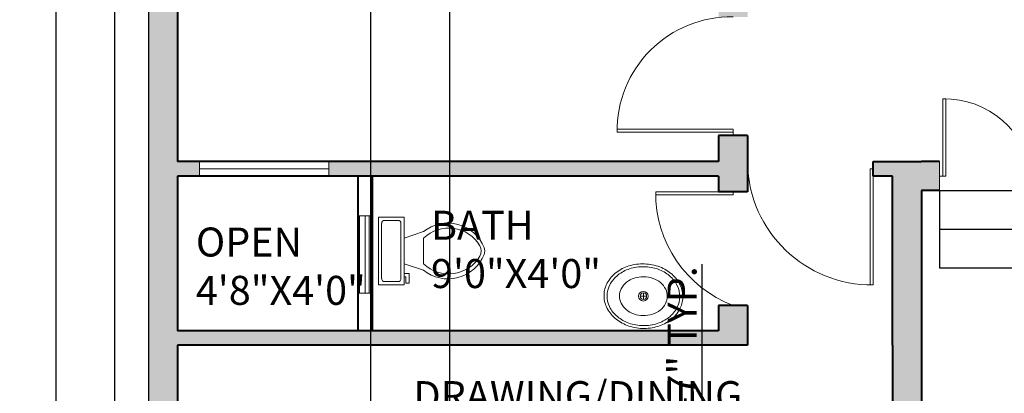
# Model space of a CAD drawing. Units: inches. Extents: x 1967493 to 1968177, y 907234 to 908105.
# Tile 2 of 5: x 1967549 to 1967854, y 907460 to 907576. Entities that reach past the tile are written whole.
import ezdxf

# ---------------------------------------------------------------- set-up
doc = ezdxf.new("R2010")
doc.units = ezdxf.units.IN
doc.linetypes.add('ACAD_ISO02W100', pattern=[15, 12, -3])
for name, color, linetype, lineweight in [('A-ANNO-DIMS', 2, 'Continuous', 18), ('A-AREA-IDEN', 7, 'Continuous', 25), ('A-DOOR', 3, 'Continuous', 20), ('A-FLOR-FIXT', 9, 'Continuous', 18), ('A-FLOR-STRS', 7, 'Continuous', 25), ('A-GLAZ', 4, 'Continuous', 18), ('A-WALL', 7, 'Continuous', 40), ('A-WALL-OVHD', 7, 'ACAD_ISO02W100', 18), ('C-PROP', 7, 'Continuous', 25)]:
    doc.layers.add(name, color=color, linetype=linetype, lineweight=lineweight)
doc.layers.add('A-WALL-PATT', color=18, linetype='Continuous', lineweight=13, true_color=0x000000)
doc.styles.get("Standard").update_dxf_attribs({"font": 'arial.ttf'})
doc.dimstyles.new('ISO-25', dxfattribs={"dimtxt": 9, "dimasz": 9, "dimexe": 1.25, "dimexo": 0.625, "dimtad": 1, "dimdec": 1, "dimrnd": 9, "dimlunit": 3, "dimtxsty": 'Standard', "dimcen": 2.5, "dimadec": 0, "dimazin": 0, "dimtfac": 1, "dimtdec": 1, "dimtmove": 0, "dimatfit": 3, "dimfxl": 1, "dimarcsym": 0})

# ---------------------------------------------------------------- blocks, each defined once
blk = doc.blocks.new('Sink - Oval top')
for p, q in [((-1, 0), (1, 0)), ((0, 1), (0, -1))]:
    blk.add_line(p, q)
for points in [[(-12.23, 0.39, 0.117634), (-11.46, -3.36, 0.104469), (-8.88, -6.8, 0.090016), (-5.08, -9.07, 0.08192), (-0.32, -10.02, 0.08192), (4.49, -9.38, 0.090016), (8.42, -7.36, 0.104469), (11.22, -4.09, 0.117634), (12.23, -0.39, 0.117634), (11.46, 3.36, 0.104469), (8.88, 6.8, 0.090016), (5.08, 9.07, 0.08192), (0.32, 10.02, 0.08192), (-4.49, 9.38, 0.090016), (-8.42, 7.36, 0.104469), (-11.22, 4.09, 0.117634)], [(-11.29, 0.16, 0.118622), (-10.52, -3.25, 0.104678), (-8.07, -6.36, 0.089562), (-4.54, -8.37, 0.081185), (-0.13, -9.15, 0.081185), (4.3, -8.49, 0.089562), (7.89, -6.58, 0.104678), (10.42, -3.55, 0.118622), (11.29, -0.16, 0.118622), (10.52, 3.25, 0.104678), (8.07, 6.36, 0.089562), (4.54, 8.37, 0.081185), (0.13, 9.15, 0.081185), (-4.3, 8.49, 0.089562), (-7.89, 6.58, 0.104678), (-10.42, 3.55, 0.118622)], [(-7.42, 0.08, 0.118283), (-6.91, -2.17, 0.104607), (-5.29, -4.21, 0.089718), (-2.97, -5.53, 0.081436), (-0.07, -6.04, 0.081436), (2.84, -5.59, 0.089718), (5.2, -4.33, 0.104607), (6.86, -2.32, 0.118283), (7.42, -0.08, 0.118283), (6.91, 2.17, 0.104607), (5.29, 4.21, 0.089718), (2.97, 5.53, 0.081436), (0.07, 6.04, 0.081436), (-2.84, 5.59, 0.089718), (-5.2, 4.33, 0.104607), (-6.86, 2.32, 0.118283)]]:
    blk.add_lwpolyline(points, format="xyb", close=True)
for radius in [1.5, 1]:
    blk.add_circle((0, 0), radius)
blk = doc.blocks.new('Toilet - top')
for p, q in [((9.5, -6), (9.5, -2)), ((-10, -8.5), (-8, -8.5)), ((-10, -9.5), (-10, -8.5)), ((-8, -8.5), (-8, -8)), ((-7, -8), (-7, -9.5)), ((-4, -8), (-6, -14)), ((4, -8), (6, -14)), ((-7, -9.5), (-10, -9.5)), ((4, -14), (-4, -14))]:
    blk.add_line(p, q)
blk.add_lwpolyline([(10.5, -8), (10.5, 0), (-10.5, 0), (-10.5, -8)], close=True)
for points in [[(-9.5, -2), (-9.5, -6)], [(8.5, -1), (-8.5, -1)], [(-8.5, -7), (8.5, -7)]]:
    blk.add_lwpolyline(points)
for centre, radius, start, end in [((-8.62, -1.88), 0.884, 81.8699, 188.1301), ((8.62, -1.88), 0.884, 351.8699, 98.1301), ((-8.62, -6.12), 0.884, 171.8699, 278.1301), ((8.62, -6.12), 0.884, 261.8699, 8.1301), ((3.52, -21.58), 12.17, 141.4691, 247.9714), ((4.2, -21.82), 11.33, 136.3677, 238.9468), ((-3.52, -21.58), 12.17, 292.0284, 38.5307), ((-4.2, -21.82), 11.33, 301.053, 43.6321), ((0, -27.88), 4, 245.7318, 294.2682), ((0, -29), 4, 254.8605, 285.1395)]:
    blk.add_arc(centre, radius, start, end)
blk = doc.blocks.new('*D12')
at = {"layer": 'A-ANNO-DIMS', "color": 0, "lineweight": -2, "transparency": 16777216}
for p, q in [((1967588.15, 908000.17), (1967558.93, 908000.17)), ((1967560.18, 907289.17), (1967560.18, 907991.17)), ((1967588.15, 907280.17), (1967558.93, 907280.17))]:
    blk.add_line(p, q, dxfattribs=at)
at = {"layer": 'A-ANNO-DIMS', "color": 0, "transparency": 16777216}
for points in [[(1967558.68, 907991.17), (1967561.68, 907991.17), (1967560.18, 908000.17)], [(1967558.68, 907289.17), (1967561.68, 907289.17), (1967560.18, 907280.17)]]:
    blk.add_solid(points, dxfattribs=at)
at = {"layer": 'Defpoints', "color": 0, "transparency": 16777216}
for p in [(1967560.18, 908000.17), (1967588.78, 908000.17), (1967588.78, 907280.17)]:
    blk.add_point(p, dxfattribs=at)
at = {"layer": 'A-ANNO-DIMS', "color": 0, "transparency": 16777216, "insert": (1967554.96, 907640.17), "char_height": 9, "attachment_point": 5, "rotation": 90}
blk.add_mtext("60'", dxfattribs=at)
blk = doc.blocks.new('*D13')
at = {"layer": 'A-ANNO-DIMS', "color": 0, "lineweight": -2, "transparency": 16777216}
for p, q in [((1967588.15, 908000.17), (1967577.16, 908000.17)), ((1967578.41, 907343.17), (1967578.41, 907991.17)), ((1967588.15, 907334.17), (1967577.16, 907334.17))]:
    blk.add_line(p, q, dxfattribs=at)
at = {"layer": 'A-ANNO-DIMS', "color": 0, "transparency": 16777216}
for points in [[(1967576.91, 907991.17), (1967579.91, 907991.17), (1967578.41, 908000.17)], [(1967576.91, 907343.17), (1967579.91, 907343.17), (1967578.41, 907334.17)]]:
    blk.add_solid(points, dxfattribs=at)
at = {"layer": 'Defpoints', "color": 0, "transparency": 16777216}
for p in [(1967578.41, 908000.17), (1967588.78, 908000.17), (1967588.78, 907334.17)]:
    blk.add_point(p, dxfattribs=at)
at = {"layer": 'A-ANNO-DIMS', "color": 0, "transparency": 16777216, "insert": (1967573.19, 907667.17), "char_height": 9, "attachment_point": 5, "rotation": 90}
blk.add_mtext('55\'-6"', dxfattribs=at)
blk = doc.blocks.new('*D33')
at = {"layer": 'A-ANNO-DIMS', "color": 0, "lineweight": -2, "transparency": 16777216}
for p, q in [((1967760.75, 907435.1), (1967760.75, 907500.36)), ((1967752.38, 907435.1), (1967762, 907435.1)), ((1967760.75, 907413.1), (1967760.75, 907426.1)), ((1967752.38, 907404.1), (1967762, 907404.1))]:
    blk.add_line(p, q, dxfattribs=at)
at = {"layer": 'A-ANNO-DIMS', "color": 0, "transparency": 16777216}
for points in [[(1967759.25, 907426.1), (1967762.25, 907426.1), (1967760.75, 907435.1)], [(1967759.25, 907413.1), (1967762.25, 907413.1), (1967760.75, 907404.1)]]:
    blk.add_solid(points, dxfattribs=at)
at = {"layer": 'Defpoints', "color": 0, "transparency": 16777216}
for p in [(1967751.75, 907435.1), (1967760.75, 907435.1), (1967751.75, 907404.1)]:
    blk.add_point(p, dxfattribs=at)
at = {"layer": 'A-ANNO-DIMS', "color": 0, "transparency": 16777216, "insert": (1967755.61, 907472.23), "char_height": 9, "attachment_point": 5, "rotation": 90}
blk.add_mtext('2\'-7" TYP.', dxfattribs=at)
blk = doc.blocks.new('*D52')
at = {"layer": 'A-ANNO-DIMS', "color": 0, "lineweight": -2, "transparency": 16777216}
for p, q in [((1967657.78, 907720.78), (1967657.78, 907240.77)), ((1967682.26, 907720.78), (1967682.26, 907240.77)), ((1967666.78, 907242.02), (1967673.26, 907242.02)), ((1967682.26, 907242.02), (1967737.56, 907242.02))]:
    blk.add_line(p, q, dxfattribs=at)
at = {"layer": 'A-ANNO-DIMS', "color": 0, "transparency": 16777216}
for points in [[(1967666.78, 907243.52), (1967666.78, 907240.52), (1967657.78, 907242.02)], [(1967673.26, 907243.52), (1967673.26, 907240.52), (1967682.26, 907242.02)]]:
    blk.add_solid(points, dxfattribs=at)
at = {"layer": 'Defpoints', "color": 0, "transparency": 16777216}
for p in [(1967657.78, 907721.4), (1967682.26, 907721.4), (1967682.26, 907242.02)]:
    blk.add_point(p, dxfattribs=at)
at = {"layer": 'A-ANNO-DIMS', "color": 0, "transparency": 16777216, "insert": (1967714.41, 907247.29), "char_height": 9, "attachment_point": 5}
blk.add_mtext('2\'-0 1/2"', dxfattribs=at)

msp = doc.modelspace()

# ---------------------------------------------------------------- hatches: boundary and pattern name
at = {"layer": 'A-WALL-PATT'}
h = msp.add_hatch(color=256, dxfattribs=at)
h.dxf.hatch_style = 1
h.paths.add_polyline_path([(1967597.78, 907991.17), (1967717.78, 907991.17), (1967717.78, 907980.85), (1967726.78, 907980.85), (1967726.78, 907991.17), (1967885.78, 907991.17), (1967885.78, 907978.94), (1967894.78, 907978.94), (1967894.78, 907991.17), (1968059.78, 907991.17), (1968059.78, 907943.17), (1968039.39, 907943.17), (1968039.39, 907934.17), (1968059.78, 907934.17), (1968059.78, 907790.17), (1968052.82, 907790.17), (1968052.82, 907781.17), (1968059.78, 907781.17), (1968059.78, 907635.17), (1968052.82, 907635.17), (1968052.82, 907626.17), (1968059.78, 907626.17), (1968059.78, 907532.17), (1967892.06, 907532.17), (1967892.06, 907523.17), (1967951.97, 907523.17), (1967951.97, 907525.77), (1968004.23, 907525.77), (1968004.23, 907523.17), (1968059.78, 907523.17), (1968059.78, 907280.17), (1968068.78, 907280.17), (1968068.78, 908000.17), (1967588.78, 908000.17), (1967588.78, 907334.17), (1967828.78, 907334.17), (1967828.78, 907349.71), (1967819.78, 907349.71), (1967819.78, 907343.17), (1967597.78, 907343.17), (1967597.78, 907475.17), (1967774.78, 907475.17), (1967774.78, 907487.51), (1967765.78, 907487.51), (1967765.78, 907479.67), (1967597.78, 907479.67), (1967597.78, 907527.67), (1967604.66, 907527.67), (1967604.66, 907532.17), (1967597.78, 907532.17), (1967597.78, 907790.17), (1967597.78, 907934.17), (1967607.68, 907934.17), (1967607.68, 907943.17), (1967597.78, 907943.17)])
h.paths.add_polyline_path([(1967726.78, 907956.85), (1967717.78, 907956.85), (1967717.78, 907943.17), (1967726.78, 907943.17)], flags=17)
h.paths.add_polyline_path([(1967731.77, 907943.17), (1967651.01, 907943.17), (1967639.17, 907943.17), (1967639.17, 907934.17), (1967651.01, 907934.17), (1967731.77, 907934.17)], flags=17)
h.paths.add_polyline_path([(1967810.78, 907895.17), (1967774.78, 907895.17), (1967774.78, 907903.7), (1967765.78, 907903.7), (1967765.78, 907849.82), (1967765.78, 907834.76), (1967774.78, 907834.76), (1967774.78, 907849.82), (1967774.78, 907886.17), (1967810.78, 907886.17)], flags=17)
h.paths.add_polyline_path([(1967855.78, 907903.7), (1967846.78, 907903.7), (1967846.78, 907895.17), (1967845.59, 907895.17), (1967845.59, 907886.17), (1967846.78, 907886.17), (1967846.78, 907849.82), (1967846.78, 907834.76), (1967855.78, 907834.76), (1967855.78, 907849.82)], flags=17)
h.paths.add_polyline_path([(1968003.67, 907943.17), (1967999.78, 907943.17), (1967999.78, 907946.67), (1967990.78, 907946.67), (1967990.78, 907943.17), (1967881.11, 907943.17), (1967881.11, 907934.17), (1968003.67, 907934.17)], flags=17)
h.paths.add_polyline_path([(1967999.78, 907991.17), (1967990.78, 907991.17), (1967990.78, 907969.75, -0.052013), (1967995.28, 907969.73), (1967999.78, 907969.73)], flags=17)
h.paths.add_polyline_path([(1967777.59, 907790.17), (1967774.78, 907790.17), (1967774.78, 907796.26), (1967765.78, 907796.26), (1967765.78, 907790.17), (1967648.78, 907790.17), (1967648.78, 907769.17), (1967597.78, 907769.17), (1967597.78, 907760.17), (1967648.78, 907760.17), (1967648.78, 907749.33), (1967657.78, 907749.33), (1967657.78, 907781.17), (1967765.78, 907781.17), (1967765.78, 907721), (1967774.78, 907721), (1967774.78, 907781.17), (1967777.59, 907781.17)], flags=17)
h.paths.add_polyline_path([(1968016.82, 907790.17), (1967855.78, 907790.17), (1967855.78, 907796.26), (1967846.78, 907796.26), (1967846.78, 907790.17), (1967843.5, 907790.17), (1967843.5, 907781.17), (1967855.78, 907781.17), (1968002.78, 907781.17), (1968002.78, 907767.09), (1968011.78, 907767.09), (1968011.78, 907781.17), (1968016.82, 907781.17)], flags=17)
h.paths.add_polyline_path([(1968011.78, 907731.09), (1968002.78, 907731.09), (1968002.78, 907698.5), (1968011.78, 907698.5)], flags=17)
h.paths.add_polyline_path([(1968011.78, 907662.5), (1968002.78, 907662.5), (1968002.78, 907635.17), (1967892.06, 907635.17), (1967892.06, 907626.17), (1968016.82, 907626.17), (1968016.82, 907635.17), (1968011.78, 907635.17)], flags=17)
h.paths.add_polyline_path([(1967774.78, 907679.04), (1967765.78, 907679.04), (1967765.78, 907673.17), (1967657.78, 907673.17), (1967657.78, 907679.08), (1967648.78, 907679.08), (1967648.78, 907673.17), (1967639.33, 907673.17), (1967639.33, 907664.17), (1967765.78, 907664.17), (1967765.78, 907577.1), (1967768.96, 907577.1, -0.009361), (1967770.28, 907577.1), (1967774.78, 907577.1), (1967774.78, 907626.17), (1967779.99, 907626.17), (1967779.99, 907635.17), (1967774.78, 907635.17)], flags=17)
h.paths.add_polyline_path([(1967603.33, 907673.17), (1967597.78, 907673.17), (1967597.78, 907664.17), (1967603.33, 907664.17)], flags=17)
h.paths.add_polyline_path([(1967774.78, 907540.27), (1967765.78, 907540.27), (1967765.78, 907532.17), (1967644.82, 907532.17), (1967644.82, 907527.67), (1967765.78, 907527.67), (1967765.78, 907522.83), (1967774.78, 907522.83)], flags=17)
h.paths.add_polyline_path([(1967828.78, 907475.17), (1967828.78, 907479.67), (1967828.78, 907523.17), (1967834.39, 907523.17), (1967834.39, 907532.17), (1967828.78, 907532.17), (1967813.83, 907532.17), (1967813.83, 907527.67), (1967819.78, 907527.67), (1967819.78, 907479.67), (1967819.78, 907475.17), (1967819.78, 907388.61), (1967828.78, 907388.61)], flags=17)

# ---------------------------------------------------------------- linework, layer by layer
at = {"layer": 'A-DOOR'}
for p, q in [((1967835.39, 907527.67), (1967835.39, 907551.67)), ((1967835.39, 907551.67), (1967836.39, 907551.67)), ((1967836.39, 907551.67), (1967836.39, 907527.67)), ((1967734.28, 907541.27), (1967734.28, 907542.27)), ((1967734.28, 907542.27), (1967770.28, 907542.27)), ((1967770.28, 907541.27), (1967734.28, 907541.27)), ((1967770.28, 907542.27), (1967770.28, 907541.27)), ((1967770.28, 907540.27), (1967770.28, 907541.27)), ((1967813.83, 907529.92), (1967812.83, 907529.92)), ((1967812.83, 907529.92), (1967812.83, 907493.92)), ((1967813.83, 907493.92), (1967813.83, 907527.67)), ((1967834.39, 907527.67), (1967835.39, 907527.67)), ((1967836.39, 907527.67), (1967835.39, 907527.67)), ((1967746.28, 907521.83), (1967746.28, 907522.83)), ((1967746.28, 907522.83), (1967765.78, 907522.83)), ((1967770.28, 907522.83), (1967770.28, 907521.83)), ((1967770.28, 907521.83), (1967746.28, 907521.83)), ((1967812.83, 907493.92), (1967813.83, 907493.92))]:
    msp.add_line(p, q, dxfattribs=at)
for centre, radius, start, end in [((1967769.62, 907541.77), 35.34, 88.9273, 180.8106), ((1967835.89, 907524.1), 27.57, 7.4241, 91.0393), ((1967813.33, 907532.47), 38.56, 181.3689, 270.743), ((1967783.54, 907522.33), 37.26, 179.2311, 249.1587)]:
    msp.add_arc(centre, radius, start, end, dxfattribs=at)
at = {"layer": 'A-FLOR-STRS'}
for p, q in [((1967834.39, 907523.17), (1967892.06, 907523.17)), ((1967834.39, 907523.17), (1967834.39, 907499.17)), ((1967834.39, 907511.17), (1967892.06, 907511.17)), ((1967834.39, 907499.17), (1967892.06, 907499.17))]:
    msp.add_line(p, q, dxfattribs=at)
at = {"layer": 'A-GLAZ'}
for p, q in [((1967604.66, 907532.17), (1967604.66, 907527.67)), ((1967644.82, 907532.17), (1967644.82, 907527.67)), ((1967604.66, 907529.92), (1967644.82, 907529.92)), ((1967653.78, 907515.38), (1967658.28, 907515.38)), ((1967654.37, 907515.38), (1967654.37, 907491.38)), ((1967656.03, 907515.38), (1967656.03, 907491.38)), ((1967657.37, 907515.38), (1967657.37, 907491.38)), ((1967653.78, 907491.38), (1967658.28, 907491.38))]:
    msp.add_line(p, q, dxfattribs=at)
at = {"layer": 'A-WALL'}
for p, q in [((1967597.78, 907790.17), (1967597.78, 907532.17)), ((1967774.78, 907540.27), (1967765.78, 907540.27)), ((1967765.78, 907540.27), (1967765.78, 907532.17)), ((1967774.78, 907540.27), (1967774.78, 907522.83)), ((1967765.78, 907532.17), (1967597.78, 907532.17)), ((1967813.83, 907527.67), (1967813.83, 907532.17)), ((1967813.83, 907532.17), (1967828.78, 907532.17)), ((1967834.39, 907532.17), (1967828.78, 907532.17)), ((1967765.78, 907527.67), (1967597.78, 907527.67)), ((1967597.78, 907527.67), (1967597.78, 907479.67)), ((1967653.78, 907527.67), (1967653.78, 907479.67)), ((1967658.28, 907527.67), (1967658.28, 907479.67)), ((1967765.78, 907527.67), (1967765.78, 907522.83)), ((1967819.78, 907527.67), (1967813.83, 907527.67)), ((1967819.78, 907479.67), (1967819.78, 907527.67)), ((1967774.78, 907522.83), (1967765.78, 907522.83)), ((1967828.78, 907523.17), (1967828.78, 907479.67)), ((1967834.39, 907523.17), (1967828.78, 907523.17)), ((1967774.78, 907487.51), (1967765.78, 907487.51)), ((1967765.78, 907487.51), (1967765.78, 907479.67)), ((1967774.78, 907487.51), (1967774.78, 907475.17)), ((1967765.78, 907479.67), (1967597.78, 907479.67)), ((1967819.78, 907475.17), (1967819.78, 907479.67)), ((1967828.78, 907479.67), (1967828.78, 907475.17)), ((1967774.78, 907475.17), (1967597.78, 907475.17)), ((1967597.78, 907475.17), (1967597.78, 907343.17)), ((1967819.78, 907475.17), (1967819.78, 907388.61)), ((1967828.78, 907475.17), (1967828.78, 907334.17))]:
    msp.add_line(p, q, dxfattribs=at)
at = {"layer": 'A-WALL-OVHD'}
msp.add_line((1967834.39, 907532.17), (1967834.39, 907523.17), dxfattribs=at)
at = {"layer": 'C-PROP'}
msp.add_line((1967588.78, 908000.17), (1967588.78, 907280.17), dxfattribs=at)

# ---------------------------------------------------------------- block references
at = {"layer": 'A-FLOR-FIXT', "rotation": 89.99999999999999}
msp.add_blockref('Toilet - top', (1967660.2, 907504.43), dxfattribs=at)
at = {"layer": 'A-FLOR-FIXT'}
msp.add_blockref('Sink - Oval top', (1967742.46, 907490.4), dxfattribs=at)

# ---------------------------------------------------------------- texts
at = {"layer": 'A-AREA-IDEN', "char_height": 9, "attachment_point": 1}
for s, width, heights, insert in [('BATH\\P9\'0"X4\'0"', 56.0747, [24.74], (1967676.53, 907516.92)), ('OPEN\\P4\'8"X4\'0"', 56.0747, [0], (1967603.52, 907511.71)), ('DRAWING/DINING\\P18\'6"X11\'0"', 158.9597, [0], (1967671.08, 907464.02))]:
    msp.add_mtext_dynamic_manual_height_columns(s, width=width, gutter_width=12.5, heights=heights, dxfattribs=dict(at, insert=insert))

# ---------------------------------------------------------------- dimensions: what is measured, and where the dimension line sits
at = {"layer": 'A-ANNO-DIMS'}
for base, p1, picture, middle in [((1967560.18, 908000.17), (1967588.78, 907280.17), '*D12', (1967554.96, 907640.17)), ((1967578.41, 908000.17), (1967588.78, 907334.17), '*D13', (1967573.19, 907667.17))]:
    dim = msp.add_linear_dim(base=base, p1=p1, p2=(1967588.78, 908000.17), angle=90, dimstyle='ISO-25', override={"dimclrd": 0, "dimclre": 0, "dimclrt": 0}, dxfattribs=at)
    dim.commit()
    dim.dimension.update_dxf_attribs({"geometry": picture, "text_midpoint": middle})
dim = msp.add_linear_dim(base=(1967682.26, 907242.02), p1=(1967657.78, 907721.4), p2=(1967682.26, 907721.4), dimstyle='ISO-25', override={"dimdec": 1, "dimlfac": 1, "dimrnd": 0, "dimzin": 1, "dimdsep": 46, "dimlunit": 4, "dimfrac": 2}, dxfattribs=at)
dim.commit()
dim.dimension.update_dxf_attribs({"geometry": '*D52', "text_midpoint": (1967714.41, 907247.29)})
dim = msp.add_linear_dim(base=(1967760.75, 907435.1), p1=(1967751.75, 907404.1), p2=(1967751.75, 907435.1), angle=90, text='<> TYP.', dimstyle='ISO-25', override={"dimdec": 1, "dimlfac": 1, "dimrnd": 0, "dimzin": 1, "dimdsep": 46, "dimlunit": 4, "dimfrac": 2}, dxfattribs=at)
dim.commit()
dim.dimension.update_dxf_attribs({"geometry": '*D33', "text_midpoint": (1967755.61, 907472.23)})

doc.saveas('drawing.dxf')
